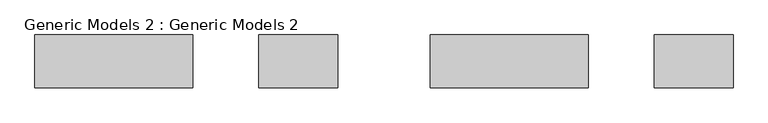
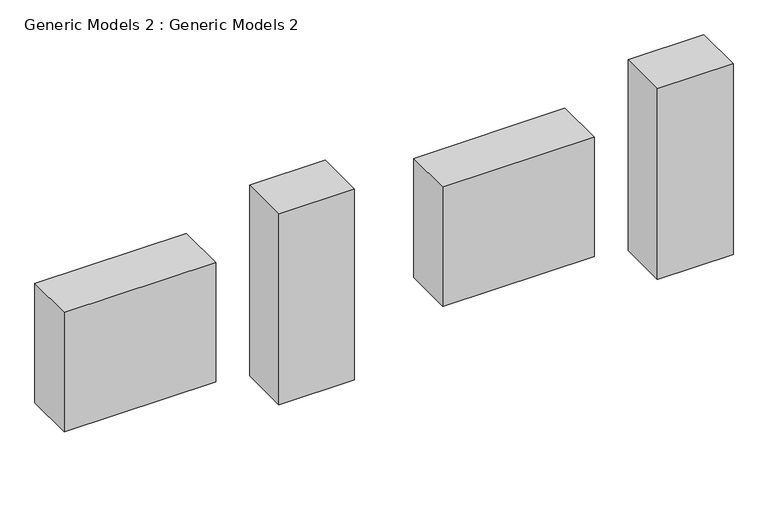
"""IFC4 building model written with IfcOpenShell, lengths in millimetres: proxy geometry, Generic Models 2 : Generic Models 2."""

from ifc_helpers import new_model, si_unit, frame, origin, place, context, project, spatial, polyline, outline, extrude, source, transform, mapped, element, save


def generic_models_2_generic_models_2_eb82d3b8(model_context):
    return source(origin(), model_context, "Body", "SweptSolid", [
        extrude(outline(polyline([(2001.4218454, -10043.743996), (1087.0218454, -10043.743996), (1087.0218454, -9738.943996), (2001.4218454, -9738.943996), (2001.4218454, -10043.743996)])), frame((0.0, 0.0, 349.8869284), z_axis=(0.0, 0.0, 1.0), x_axis=(1.0, 0.0, 0.0)), (0.0, 0.0, 1.0), 762.0),
        extrude(outline(polyline([(2840.5084916, -10043.743996), (2383.3084916, -10043.743996), (2383.3084916, -9738.943996), (2840.5084916, -9738.943996), (2840.5084916, -10043.743996)])), frame((0.0, 0.0, 67.7718225), z_axis=(0.0, 0.0, 1.0), x_axis=(1.0, 0.0, 0.0)), (0.0, 0.0, 1.0), 1219.2),
        extrude(outline(polyline([(4287.4218454, -10043.743996), (3373.0218454, -10043.743996), (3373.0218454, -9738.943996), (4287.4218454, -9738.943996), (4287.4218454, -10043.743996)])), frame((0.0, 0.0, 349.8869284), z_axis=(0.0, 0.0, 1.0), x_axis=(1.0, 0.0, 0.0)), (0.0, 0.0, 1.0), 762.0),
        extrude(outline(polyline([(5126.5084916, -10043.743996), (4669.3084916, -10043.743996), (4669.3084916, -9738.943996), (5126.5084916, -9738.943996), (5126.5084916, -10043.743996)])), frame((0.0, 0.0, 67.7718225), z_axis=(0.0, 0.0, 1.0), x_axis=(1.0, 0.0, 0.0)), (0.0, 0.0, 1.0), 1219.2),
    ])


if __name__ == "__main__":
    model = new_model("IFC4")
    model_context = context("Model", 3, world=origin())
    ifc_project = project(units=[si_unit("LENGTHUNIT", "METRE", prefix="MILLI")], contexts=[model_context])
    site = spatial("IfcSite", under=ifc_project)
    building = spatial("IfcBuilding", under=site)
    placement = place(None, origin())
    generic_models_2_generic_models_2_shape = generic_models_2_generic_models_2_eb82d3b8(model_context)
    element("IfcBuildingElementProxy", 1, Name="Generic Models 2 : Generic Models 2", ObjectType="Generic Models 2 : Generic Models 2", at=placement, inside=building, context=model_context, shape_type="MappedRepresentation", body=[
        mapped(generic_models_2_generic_models_2_shape, transform((0.0, 0.0, 0.0), x_axis=(1.0, 0.0, 0.0), y_axis=(0.0, 1.0, 0.0), z_axis=(0.0, 0.0, 1.0))),
    ])
    save(model, "model.ifc")

# Revit data of these elements
# Element 1 (IfcBuildingElementProxy, "Generic Models 2 : Generic Models 2")
#   Materials on its faces: "Brick, Common"
# Materials
#   "Brick, Common": class "Masonry", colour RGB 170 98 104, transparency 0, Description = "Common brick", Cost = 0
